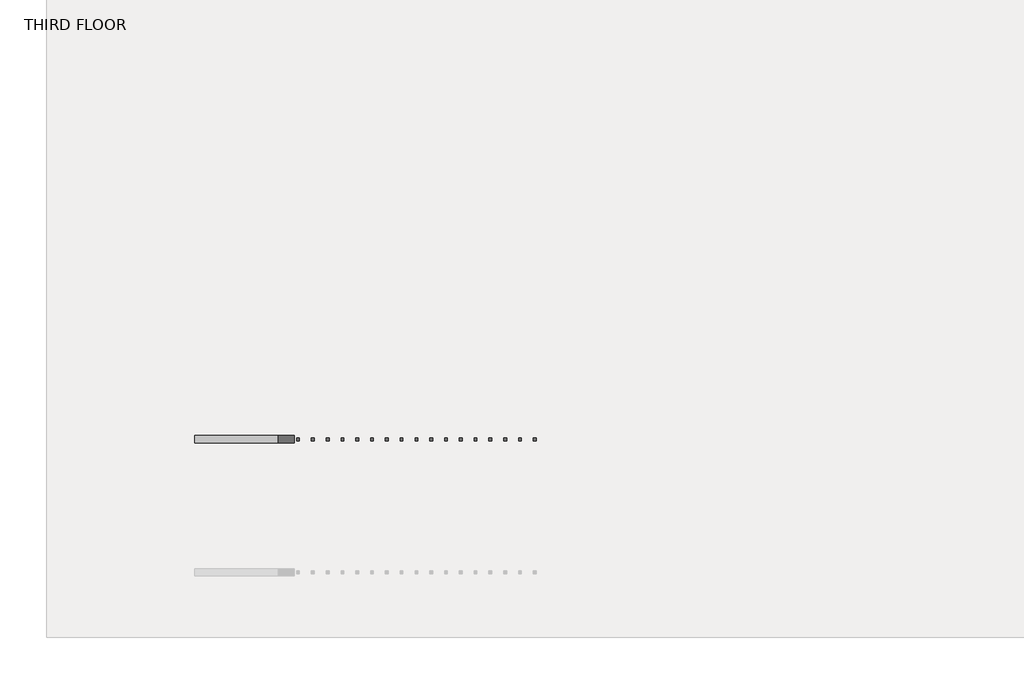
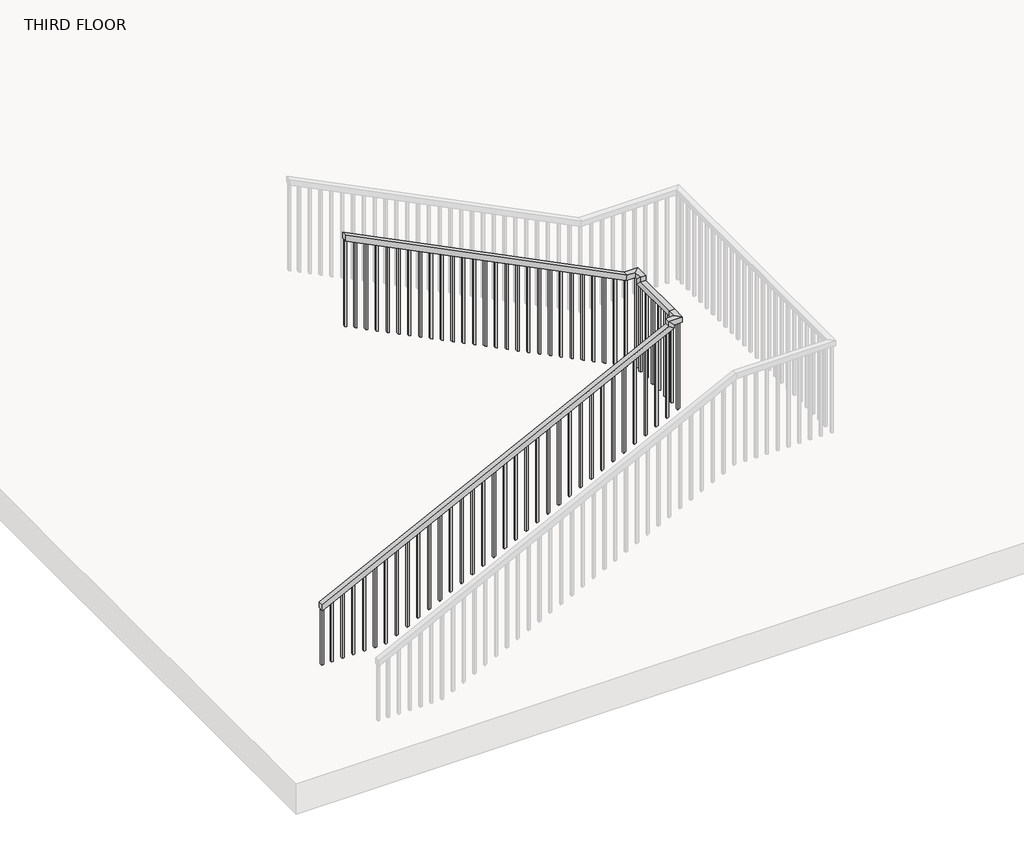
# One storey, part 2 of 2: 1 railing.
"""IFC4 building model written with IfcOpenShell, lengths in millimetres."""

from ifc_helpers import new_model, si_unit, frame, origin, place, context, project, spatial, polyline, outline, extrude, faceted_brep, element, save

model = new_model("IFC4")

# Units and contexts
model_context = context("Model", 3, world=origin())
ifc_project = project(units=[si_unit("LENGTHUNIT", "METRE", prefix="MILLI")], contexts=[model_context])

# Site, building, storey
site = spatial("IfcSite", under=ifc_project)
building = spatial("IfcBuilding", under=site)
storey = spatial("IfcBuildingStorey", under=building, Name="THIRD FLOOR", Elevation=9144.0)

# Railing
placement = place(None, origin())
element("IfcRailing", 1, ObjectType="Handrail - Rectangular", at=placement, inside=storey, context=model_context, shape_type="SolidModel", body=[
    faceted_brep([(-8362.2800418, -4455.7090076, 10058.4), (-8362.2800418, -4455.7090076, 10001.6038734), (-8362.2800418, -4506.5090076, 10001.6038734), (-8362.2800418, -4506.5090076, 10058.4), (-5111.0800418, -4455.7090076, 11684.0), (-5060.2800418, -4455.7090076, 11652.6038734), (-5060.2800418, -4506.5090076, 11652.6038734), (-5111.0800418, -4506.5090076, 11684.0), (-5111.0800418, -4455.7090076, 11734.8), (-5060.2800418, -4455.7090076, 11684.0), (-5060.2800418, -4506.5090076, 11684.0), (-5111.0800418, -4506.5090076, 11734.8), (-5034.8800418, -4455.7090076, 11734.8), (-5034.8800418, -4455.7090076, 11684.0), (-4984.0800418, -4506.5090076, 11684.0), (-4984.0800418, -4506.5090076, 11734.8), (-5034.8800418, -4379.5090076, 11734.8), (-5034.8800418, -4379.5090076, 11684.0), (-4984.0800418, -4379.5090076, 11684.0), (-4984.0800418, -4379.5090076, 11734.8), (-5034.8800418, -3907.7346494, 11734.8), (-5034.8800418, -3856.9346494, 11684.0), (-4984.0800418, -3856.9346494, 11684.0), (-4984.0800418, -3907.7346494, 11734.8), (-5034.8800418, -3907.7346494, 11785.6), (-5034.8800418, -3856.9346494, 11734.8), (-4984.0800418, -3856.9346494, 11734.8), (-4984.0800418, -3907.7346494, 11785.6), (-5034.8800418, -3831.5346494, 11785.6), (-5034.8800418, -3831.5346494, 11734.8), (-4984.0800418, -3780.7346494, 11734.8), (-4984.0800418, -3780.7346494, 11785.6), (-5111.0800418, -3831.5346494, 11785.6), (-5123.072295, -3831.5346494, 11734.8), (-5123.072295, -3780.7346494, 11734.8), (-5111.0800418, -3780.7346494, 11785.6), (-7752.6800418, -3831.5346494, 13106.4), (-7752.6800418, -3780.7346494, 13106.4), (-7752.6800418, -3780.7346494, 13049.6038734), (-7752.6800418, -3831.5346494, 13049.6038734)], [[[0, 1, 2, 3]], [[1, 0, 4, 5]], [[2, 1, 5, 6]], [[3, 2, 6, 7]], [[0, 3, 7, 4]], [[5, 4, 8, 9]], [[6, 5, 9, 10]], [[7, 6, 10, 11]], [[4, 7, 11, 8]], [[9, 8, 12, 13]], [[10, 9, 13, 14]], [[11, 10, 14, 15]], [[8, 11, 15, 12]], [[13, 12, 16, 17]], [[14, 13, 17, 18]], [[15, 14, 18, 19]], [[12, 15, 19, 16]], [[17, 16, 20, 21]], [[18, 17, 21, 22]], [[19, 18, 22, 23]], [[16, 19, 23, 20]], [[21, 20, 24, 25]], [[22, 21, 25, 26]], [[23, 22, 26, 27]], [[20, 23, 27, 24]], [[25, 24, 28, 29]], [[26, 25, 29, 30]], [[27, 26, 30, 31]], [[24, 27, 31, 28]], [[29, 28, 32, 33]], [[30, 29, 33, 34]], [[31, 30, 34, 35]], [[28, 31, 35, 32]], [[36, 37, 38, 39]], [[33, 32, 36, 39]], [[34, 33, 39, 38]], [[35, 34, 38, 37]], [[32, 35, 37, 36]]]),
    extrude(outline(polyline([(12994.0413734, -7641.5550418), (13003.5663734, -7660.6050418), (12145.9625, -7660.6050418), (12136.4375, -7641.5550418), (12994.0413734, -7641.5550418)])), frame((0.0, -3815.6596494, 0.0), z_axis=(0.0, 1.0, 0.0), x_axis=(0.0, 0.0, 1.0)), (0.0, 0.0, 1.0), 19.05),
    extrude(outline(polyline([(12943.2413734, -7539.9550418), (12952.7663734, -7559.0050418), (12095.1625, -7559.0050418), (12085.6375, -7539.9550418), (12943.2413734, -7539.9550418)])), frame((0.0, -3815.6596494, 0.0), z_axis=(0.0, 1.0, 0.0), x_axis=(0.0, 0.0, 1.0)), (0.0, 0.0, 1.0), 19.05),
    extrude(outline(polyline([(12892.4413734, -7438.3550418), (12901.9663734, -7457.4050418), (12044.3625, -7457.4050418), (12034.8375, -7438.3550418), (12892.4413734, -7438.3550418)])), frame((0.0, -3815.6596494, 0.0), z_axis=(0.0, 1.0, 0.0), x_axis=(0.0, 0.0, 1.0)), (0.0, 0.0, 1.0), 19.05),
    extrude(outline(polyline([(12841.6413734, -7336.7550418), (12851.1663734, -7355.8050418), (11993.5625, -7355.8050418), (11984.0375, -7336.7550418), (12841.6413734, -7336.7550418)])), frame((0.0, -3815.6596494, 0.0), z_axis=(0.0, 1.0, 0.0), x_axis=(0.0, 0.0, 1.0)), (0.0, 0.0, 1.0), 19.05),
    extrude(outline(polyline([(12790.8413734, -7235.1550418), (12800.3663734, -7254.2050418), (11942.7625, -7254.2050418), (11933.2375, -7235.1550418), (12790.8413734, -7235.1550418)])), frame((0.0, -3815.6596494, 0.0), z_axis=(0.0, 1.0, 0.0), x_axis=(0.0, 0.0, 1.0)), (0.0, 0.0, 1.0), 19.05),
    extrude(outline(polyline([(12740.0413734, -7133.5550418), (12749.5663734, -7152.6050418), (11891.9625, -7152.6050418), (11882.4375, -7133.5550418), (12740.0413734, -7133.5550418)])), frame((0.0, -3815.6596494, 0.0), z_axis=(0.0, 1.0, 0.0), x_axis=(0.0, 0.0, 1.0)), (0.0, 0.0, 1.0), 19.05),
    extrude(outline(polyline([(12689.2413734, -7031.9550418), (12698.7663734, -7051.0050418), (11841.1625, -7051.0050418), (11831.6375, -7031.9550418), (12689.2413734, -7031.9550418)])), frame((0.0, -3815.6596494, 0.0), z_axis=(0.0, 1.0, 0.0), x_axis=(0.0, 0.0, 1.0)), (0.0, 0.0, 1.0), 19.05),
    extrude(outline(polyline([(12638.4413734, -6930.3550418), (12647.9663734, -6949.4050418), (11790.3625, -6949.4050418), (11780.8375, -6930.3550418), (12638.4413734, -6930.3550418)])), frame((0.0, -3815.6596494, 0.0), z_axis=(0.0, 1.0, 0.0), x_axis=(0.0, 0.0, 1.0)), (0.0, 0.0, 1.0), 19.05),
    extrude(outline(polyline([(12587.6413734, -6828.7550418), (12597.1663734, -6847.8050418), (11739.5625, -6847.8050418), (11730.0375, -6828.7550418), (12587.6413734, -6828.7550418)])), frame((0.0, -3815.6596494, 0.0), z_axis=(0.0, 1.0, 0.0), x_axis=(0.0, 0.0, 1.0)), (0.0, 0.0, 1.0), 19.05),
    extrude(outline(polyline([(12536.8413734, -6727.1550418), (12546.3663734, -6746.2050418), (11688.7625, -6746.2050418), (11679.2375, -6727.1550418), (12536.8413734, -6727.1550418)])), frame((0.0, -3815.6596494, 0.0), z_axis=(0.0, 1.0, 0.0), x_axis=(0.0, 0.0, 1.0)), (0.0, 0.0, 1.0), 19.05),
    extrude(outline(polyline([(12486.0413734, -6625.5550418), (12495.5663734, -6644.6050418), (11637.9625, -6644.6050418), (11628.4375, -6625.5550418), (12486.0413734, -6625.5550418)])), frame((0.0, -3815.6596494, 0.0), z_axis=(0.0, 1.0, 0.0), x_axis=(0.0, 0.0, 1.0)), (0.0, 0.0, 1.0), 19.05),
    extrude(outline(polyline([(12435.2413734, -6523.9550418), (12444.7663734, -6543.0050418), (11587.1625, -6543.0050418), (11577.6375, -6523.9550418), (12435.2413734, -6523.9550418)])), frame((0.0, -3815.6596494, 0.0), z_axis=(0.0, 1.0, 0.0), x_axis=(0.0, 0.0, 1.0)), (0.0, 0.0, 1.0), 19.05),
    extrude(outline(polyline([(12384.4413734, -6422.3550418), (12393.9663734, -6441.4050418), (11536.3625, -6441.4050418), (11526.8375, -6422.3550418), (12384.4413734, -6422.3550418)])), frame((0.0, -3815.6596494, 0.0), z_axis=(0.0, 1.0, 0.0), x_axis=(0.0, 0.0, 1.0)), (0.0, 0.0, 1.0), 19.05),
    extrude(outline(polyline([(12333.6413734, -6320.7550418), (12343.1663734, -6339.8050418), (11485.5625, -6339.8050418), (11476.0375, -6320.7550418), (12333.6413734, -6320.7550418)])), frame((0.0, -3815.6596494, 0.0), z_axis=(0.0, 1.0, 0.0), x_axis=(0.0, 0.0, 1.0)), (0.0, 0.0, 1.0), 19.05),
    extrude(outline(polyline([(12282.8413734, -6219.1550418), (12292.3663734, -6238.2050418), (11434.7625, -6238.2050418), (11425.2375, -6219.1550418), (12282.8413734, -6219.1550418)])), frame((0.0, -3815.6596494, 0.0), z_axis=(0.0, 1.0, 0.0), x_axis=(0.0, 0.0, 1.0)), (0.0, 0.0, 1.0), 19.05),
    extrude(outline(polyline([(12232.0413734, -6117.5550418), (12241.5663734, -6136.6050418), (11383.9625, -6136.6050418), (11374.4375, -6117.5550418), (12232.0413734, -6117.5550418)])), frame((0.0, -3815.6596494, 0.0), z_axis=(0.0, 1.0, 0.0), x_axis=(0.0, 0.0, 1.0)), (0.0, 0.0, 1.0), 19.05),
    extrude(outline(polyline([(12181.2413734, -6015.9550418), (12190.7663734, -6035.0050418), (11333.1625, -6035.0050418), (11323.6375, -6015.9550418), (12181.2413734, -6015.9550418)])), frame((0.0, -3815.6596494, 0.0), z_axis=(0.0, 1.0, 0.0), x_axis=(0.0, 0.0, 1.0)), (0.0, 0.0, 1.0), 19.05),
    extrude(outline(polyline([(12130.4413734, -5914.3550418), (12139.9663734, -5933.4050418), (11282.3625, -5933.4050418), (11272.8375, -5914.3550418), (12130.4413734, -5914.3550418)])), frame((0.0, -3815.6596494, 0.0), z_axis=(0.0, 1.0, 0.0), x_axis=(0.0, 0.0, 1.0)), (0.0, 0.0, 1.0), 19.05),
    extrude(outline(polyline([(12079.6413734, -5812.7550418), (12089.1663734, -5831.8050418), (11231.5625, -5831.8050418), (11222.0375, -5812.7550418), (12079.6413734, -5812.7550418)])), frame((0.0, -3815.6596494, 0.0), z_axis=(0.0, 1.0, 0.0), x_axis=(0.0, 0.0, 1.0)), (0.0, 0.0, 1.0), 19.05),
    extrude(outline(polyline([(12028.8413734, -5711.1550418), (12038.3663734, -5730.2050418), (11180.7625, -5730.2050418), (11171.2375, -5711.1550418), (12028.8413734, -5711.1550418)])), frame((0.0, -3815.6596494, 0.0), z_axis=(0.0, 1.0, 0.0), x_axis=(0.0, 0.0, 1.0)), (0.0, 0.0, 1.0), 19.05),
    extrude(outline(polyline([(11978.0413734, -5609.5550418), (11987.5663734, -5628.6050418), (11129.9625, -5628.6050418), (11120.4375, -5609.5550418), (11978.0413734, -5609.5550418)])), frame((0.0, -3815.6596494, 0.0), z_axis=(0.0, 1.0, 0.0), x_axis=(0.0, 0.0, 1.0)), (0.0, 0.0, 1.0), 19.05),
    extrude(outline(polyline([(11927.2413734, -5507.9550418), (11936.7663734, -5527.0050418), (11079.1625, -5527.0050418), (11069.6375, -5507.9550418), (11927.2413734, -5507.9550418)])), frame((0.0, -3815.6596494, 0.0), z_axis=(0.0, 1.0, 0.0), x_axis=(0.0, 0.0, 1.0)), (0.0, 0.0, 1.0), 19.05),
    extrude(outline(polyline([(11876.4413734, -5406.3550418), (11885.9663734, -5425.4050418), (11028.3625, -5425.4050418), (11018.8375, -5406.3550418), (11876.4413734, -5406.3550418)])), frame((0.0, -3815.6596494, 0.0), z_axis=(0.0, 1.0, 0.0), x_axis=(0.0, 0.0, 1.0)), (0.0, 0.0, 1.0), 19.05),
    extrude(outline(polyline([(11825.6413734, -5304.7550418), (11835.1663734, -5323.8050418), (10977.5625, -5323.8050418), (10968.0375, -5304.7550418), (11825.6413734, -5304.7550418)])), frame((0.0, -3815.6596494, 0.0), z_axis=(0.0, 1.0, 0.0), x_axis=(0.0, 0.0, 1.0)), (0.0, 0.0, 1.0), 19.05),
    extrude(outline(polyline([(11774.8413734, -5203.1550418), (11784.3663734, -5222.2050418), (10926.7625, -5222.2050418), (10917.2375, -5203.1550418), (11774.8413734, -5203.1550418)])), frame((0.0, -3815.6596494, 0.0), z_axis=(0.0, 1.0, 0.0), x_axis=(0.0, 0.0, 1.0)), (0.0, 0.0, 1.0), 19.05),
    extrude(outline(polyline([(11734.8, -5101.5550418), (11734.8, -5120.6050418), (10875.9625, -5120.6050418), (10866.4375, -5101.5550418), (11734.8, -5101.5550418)])), frame((0.0, -3815.6596494, 0.0), z_axis=(0.0, 1.0, 0.0), x_axis=(0.0, 0.0, 1.0)), (0.0, 0.0, 1.0), 19.05),
    extrude(outline(polyline([(-4999.9550418, -3881.0340076), (-5019.0050418, -3881.0340076), (-5019.0050418, -3861.9840076), (-4999.9550418, -3861.9840076), (-4999.9550418, -3881.0340076)])), frame((0.0, 0.0, 10820.4), z_axis=(0.0, 0.0, 1.0), x_axis=(1.0, 0.0, 0.0)), (0.0, 0.0, 1.0), 863.6),
    extrude(outline(polyline([(-4999.9550418, -3982.6340076), (-5019.0050418, -3982.6340076), (-5019.0050418, -3963.5840076), (-4999.9550418, -3963.5840076), (-4999.9550418, -3982.6340076)])), frame((0.0, 0.0, 10820.4), z_axis=(0.0, 0.0, 1.0), x_axis=(1.0, 0.0, 0.0)), (0.0, 0.0, 1.0), 863.6),
    extrude(outline(polyline([(-4999.9550418, -4084.2340076), (-5019.0050418, -4084.2340076), (-5019.0050418, -4065.1840076), (-4999.9550418, -4065.1840076), (-4999.9550418, -4084.2340076)])), frame((0.0, 0.0, 10820.4), z_axis=(0.0, 0.0, 1.0), x_axis=(1.0, 0.0, 0.0)), (0.0, 0.0, 1.0), 863.6),
    extrude(outline(polyline([(-4999.9550418, -4185.8340076), (-5019.0050418, -4185.8340076), (-5019.0050418, -4166.7840076), (-4999.9550418, -4166.7840076), (-4999.9550418, -4185.8340076)])), frame((0.0, 0.0, 10820.4), z_axis=(0.0, 0.0, 1.0), x_axis=(1.0, 0.0, 0.0)), (0.0, 0.0, 1.0), 863.6),
    extrude(outline(polyline([(-4999.9550418, -4287.4340076), (-5019.0050418, -4287.4340076), (-5019.0050418, -4268.3840076), (-4999.9550418, -4268.3840076), (-4999.9550418, -4287.4340076)])), frame((0.0, 0.0, 10820.4), z_axis=(0.0, 0.0, 1.0), x_axis=(1.0, 0.0, 0.0)), (0.0, 0.0, 1.0), 863.6),
    extrude(outline(polyline([(-4999.9550418, -4389.0340076), (-5019.0050418, -4389.0340076), (-5019.0050418, -4369.9840076), (-4999.9550418, -4369.9840076), (-4999.9550418, -4389.0340076)])), frame((0.0, 0.0, 10820.4), z_axis=(0.0, 0.0, 1.0), x_axis=(1.0, 0.0, 0.0)), (0.0, 0.0, 1.0), 863.6),
    extrude(outline(polyline([(11631.9663734, -5101.5550418), (11622.4413734, -5120.6050418), (10764.8375, -5120.6050418), (10774.3625, -5101.5550418), (11631.9663734, -5101.5550418)])), frame((0.0, -4490.6340076, 0.0), z_axis=(0.0, 1.0, 0.0), x_axis=(0.0, 0.0, 1.0)), (0.0, 0.0, 1.0), 19.05),
    extrude(outline(polyline([(11581.1663734, -5203.1550418), (11571.6413734, -5222.2050418), (10714.0375, -5222.2050418), (10723.5625, -5203.1550418), (11581.1663734, -5203.1550418)])), frame((0.0, -4490.6340076, 0.0), z_axis=(0.0, 1.0, 0.0), x_axis=(0.0, 0.0, 1.0)), (0.0, 0.0, 1.0), 19.05),
    extrude(outline(polyline([(11530.3663734, -5304.7550418), (11520.8413734, -5323.8050418), (10663.2375, -5323.8050418), (10672.7625, -5304.7550418), (11530.3663734, -5304.7550418)])), frame((0.0, -4490.6340076, 0.0), z_axis=(0.0, 1.0, 0.0), x_axis=(0.0, 0.0, 1.0)), (0.0, 0.0, 1.0), 19.05),
    extrude(outline(polyline([(11479.5663734, -5406.3550418), (11470.0413734, -5425.4050418), (10612.4375, -5425.4050418), (10621.9625, -5406.3550418), (11479.5663734, -5406.3550418)])), frame((0.0, -4490.6340076, 0.0), z_axis=(0.0, 1.0, 0.0), x_axis=(0.0, 0.0, 1.0)), (0.0, 0.0, 1.0), 19.05),
    extrude(outline(polyline([(11428.7663734, -5507.9550418), (11419.2413734, -5527.0050418), (10561.6375, -5527.0050418), (10571.1625, -5507.9550418), (11428.7663734, -5507.9550418)])), frame((0.0, -4490.6340076, 0.0), z_axis=(0.0, 1.0, 0.0), x_axis=(0.0, 0.0, 1.0)), (0.0, 0.0, 1.0), 19.05),
    extrude(outline(polyline([(11377.9663734, -5609.5550418), (11368.4413734, -5628.6050418), (10510.8375, -5628.6050418), (10520.3625, -5609.5550418), (11377.9663734, -5609.5550418)])), frame((0.0, -4490.6340076, 0.0), z_axis=(0.0, 1.0, 0.0), x_axis=(0.0, 0.0, 1.0)), (0.0, 0.0, 1.0), 19.05),
    extrude(outline(polyline([(11327.1663734, -5711.1550418), (11317.6413734, -5730.2050418), (10460.0375, -5730.2050418), (10469.5625, -5711.1550418), (11327.1663734, -5711.1550418)])), frame((0.0, -4490.6340076, 0.0), z_axis=(0.0, 1.0, 0.0), x_axis=(0.0, 0.0, 1.0)), (0.0, 0.0, 1.0), 19.05),
    extrude(outline(polyline([(11276.3663734, -5812.7550418), (11266.8413734, -5831.8050418), (10409.2375, -5831.8050418), (10418.7625, -5812.7550418), (11276.3663734, -5812.7550418)])), frame((0.0, -4490.6340076, 0.0), z_axis=(0.0, 1.0, 0.0), x_axis=(0.0, 0.0, 1.0)), (0.0, 0.0, 1.0), 19.05),
    extrude(outline(polyline([(11225.5663734, -5914.3550418), (11216.0413734, -5933.4050418), (10358.4375, -5933.4050418), (10367.9625, -5914.3550418), (11225.5663734, -5914.3550418)])), frame((0.0, -4490.6340076, 0.0), z_axis=(0.0, 1.0, 0.0), x_axis=(0.0, 0.0, 1.0)), (0.0, 0.0, 1.0), 19.05),
    extrude(outline(polyline([(11174.7663734, -6015.9550418), (11165.2413734, -6035.0050418), (10307.6375, -6035.0050418), (10317.1625, -6015.9550418), (11174.7663734, -6015.9550418)])), frame((0.0, -4490.6340076, 0.0), z_axis=(0.0, 1.0, 0.0), x_axis=(0.0, 0.0, 1.0)), (0.0, 0.0, 1.0), 19.05),
    extrude(outline(polyline([(11123.9663734, -6117.5550418), (11114.4413734, -6136.6050418), (10256.8375, -6136.6050418), (10266.3625, -6117.5550418), (11123.9663734, -6117.5550418)])), frame((0.0, -4490.6340076, 0.0), z_axis=(0.0, 1.0, 0.0), x_axis=(0.0, 0.0, 1.0)), (0.0, 0.0, 1.0), 19.05),
    extrude(outline(polyline([(11073.1663734, -6219.1550418), (11063.6413734, -6238.2050418), (10206.0375, -6238.2050418), (10215.5625, -6219.1550418), (11073.1663734, -6219.1550418)])), frame((0.0, -4490.6340076, 0.0), z_axis=(0.0, 1.0, 0.0), x_axis=(0.0, 0.0, 1.0)), (0.0, 0.0, 1.0), 19.05),
    extrude(outline(polyline([(11022.3663734, -6320.7550418), (11012.8413734, -6339.8050418), (10155.2375, -6339.8050418), (10164.7625, -6320.7550418), (11022.3663734, -6320.7550418)])), frame((0.0, -4490.6340076, 0.0), z_axis=(0.0, 1.0, 0.0), x_axis=(0.0, 0.0, 1.0)), (0.0, 0.0, 1.0), 19.05),
    extrude(outline(polyline([(10971.5663734, -6422.3550418), (10962.0413734, -6441.4050418), (10104.4375, -6441.4050418), (10113.9625, -6422.3550418), (10971.5663734, -6422.3550418)])), frame((0.0, -4490.6340076, 0.0), z_axis=(0.0, 1.0, 0.0), x_axis=(0.0, 0.0, 1.0)), (0.0, 0.0, 1.0), 19.05),
    extrude(outline(polyline([(10920.7663734, -6523.9550418), (10911.2413734, -6543.0050418), (10053.6375, -6543.0050418), (10063.1625, -6523.9550418), (10920.7663734, -6523.9550418)])), frame((0.0, -4490.6340076, 0.0), z_axis=(0.0, 1.0, 0.0), x_axis=(0.0, 0.0, 1.0)), (0.0, 0.0, 1.0), 19.05),
    extrude(outline(polyline([(10869.9663734, -6625.5550418), (10860.4413734, -6644.6050418), (10002.8375, -6644.6050418), (10012.3625, -6625.5550418), (10869.9663734, -6625.5550418)])), frame((0.0, -4490.6340076, 0.0), z_axis=(0.0, 1.0, 0.0), x_axis=(0.0, 0.0, 1.0)), (0.0, 0.0, 1.0), 19.05),
    extrude(outline(polyline([(10819.1663734, -6727.1550418), (10809.6413734, -6746.2050418), (9952.0375, -6746.2050418), (9961.5625, -6727.1550418), (10819.1663734, -6727.1550418)])), frame((0.0, -4490.6340076, 0.0), z_axis=(0.0, 1.0, 0.0), x_axis=(0.0, 0.0, 1.0)), (0.0, 0.0, 1.0), 19.05),
    extrude(outline(polyline([(10768.3663734, -6828.7550418), (10758.8413734, -6847.8050418), (9901.2375, -6847.8050418), (9910.7625, -6828.7550418), (10768.3663734, -6828.7550418)])), frame((0.0, -4490.6340076, 0.0), z_axis=(0.0, 1.0, 0.0), x_axis=(0.0, 0.0, 1.0)), (0.0, 0.0, 1.0), 19.05),
    extrude(outline(polyline([(10717.5663734, -6930.3550418), (10708.0413734, -6949.4050418), (9850.4375, -6949.4050418), (9859.9625, -6930.3550418), (10717.5663734, -6930.3550418)])), frame((0.0, -4490.6340076, 0.0), z_axis=(0.0, 1.0, 0.0), x_axis=(0.0, 0.0, 1.0)), (0.0, 0.0, 1.0), 19.05),
    extrude(outline(polyline([(10666.7663734, -7031.9550418), (10657.2413734, -7051.0050418), (9799.6375, -7051.0050418), (9809.1625, -7031.9550418), (10666.7663734, -7031.9550418)])), frame((0.0, -4490.6340076, 0.0), z_axis=(0.0, 1.0, 0.0), x_axis=(0.0, 0.0, 1.0)), (0.0, 0.0, 1.0), 19.05),
    extrude(outline(polyline([(10615.9663734, -7133.5550418), (10606.4413734, -7152.6050418), (9748.8375, -7152.6050418), (9758.3625, -7133.5550418), (10615.9663734, -7133.5550418)])), frame((0.0, -4490.6340076, 0.0), z_axis=(0.0, 1.0, 0.0), x_axis=(0.0, 0.0, 1.0)), (0.0, 0.0, 1.0), 19.05),
    extrude(outline(polyline([(10565.1663734, -7235.1550418), (10555.6413734, -7254.2050418), (9698.0375, -7254.2050418), (9707.5625, -7235.1550418), (10565.1663734, -7235.1550418)])), frame((0.0, -4490.6340076, 0.0), z_axis=(0.0, 1.0, 0.0), x_axis=(0.0, 0.0, 1.0)), (0.0, 0.0, 1.0), 19.05),
    extrude(outline(polyline([(10514.3663734, -7336.7550418), (10504.8413734, -7355.8050418), (9647.2375, -7355.8050418), (9656.7625, -7336.7550418), (10514.3663734, -7336.7550418)])), frame((0.0, -4490.6340076, 0.0), z_axis=(0.0, 1.0, 0.0), x_axis=(0.0, 0.0, 1.0)), (0.0, 0.0, 1.0), 19.05),
    extrude(outline(polyline([(10463.5663734, -7438.3550418), (10454.0413734, -7457.4050418), (9596.4375, -7457.4050418), (9605.9625, -7438.3550418), (10463.5663734, -7438.3550418)])), frame((0.0, -4490.6340076, 0.0), z_axis=(0.0, 1.0, 0.0), x_axis=(0.0, 0.0, 1.0)), (0.0, 0.0, 1.0), 19.05),
    extrude(outline(polyline([(10412.7663734, -7539.9550418), (10403.2413734, -7559.0050418), (9545.6375, -7559.0050418), (9555.1625, -7539.9550418), (10412.7663734, -7539.9550418)])), frame((0.0, -4490.6340076, 0.0), z_axis=(0.0, 1.0, 0.0), x_axis=(0.0, 0.0, 1.0)), (0.0, 0.0, 1.0), 19.05),
    extrude(outline(polyline([(10361.9663734, -7641.5550418), (10352.4413734, -7660.6050418), (9494.8375, -7660.6050418), (9504.3625, -7641.5550418), (10361.9663734, -7641.5550418)])), frame((0.0, -4490.6340076, 0.0), z_axis=(0.0, 1.0, 0.0), x_axis=(0.0, 0.0, 1.0)), (0.0, 0.0, 1.0), 19.05),
    extrude(outline(polyline([(10311.1663734, -7743.1550418), (10301.6413734, -7762.2050418), (9444.0375, -7762.2050418), (9453.5625, -7743.1550418), (10311.1663734, -7743.1550418)])), frame((0.0, -4490.6340076, 0.0), z_axis=(0.0, 1.0, 0.0), x_axis=(0.0, 0.0, 1.0)), (0.0, 0.0, 1.0), 19.05),
    extrude(outline(polyline([(10260.3663734, -7844.7550418), (10250.8413734, -7863.8050418), (9393.2375, -7863.8050418), (9402.7625, -7844.7550418), (10260.3663734, -7844.7550418)])), frame((0.0, -4490.6340076, 0.0), z_axis=(0.0, 1.0, 0.0), x_axis=(0.0, 0.0, 1.0)), (0.0, 0.0, 1.0), 19.05),
    extrude(outline(polyline([(10209.5663734, -7946.3550418), (10200.0413734, -7965.4050418), (9342.4375, -7965.4050418), (9351.9625, -7946.3550418), (10209.5663734, -7946.3550418)])), frame((0.0, -4490.6340076, 0.0), z_axis=(0.0, 1.0, 0.0), x_axis=(0.0, 0.0, 1.0)), (0.0, 0.0, 1.0), 19.05),
    extrude(outline(polyline([(10158.7663734, -8047.9550418), (10149.2413734, -8067.0050418), (9291.6375, -8067.0050418), (9301.1625, -8047.9550418), (10158.7663734, -8047.9550418)])), frame((0.0, -4490.6340076, 0.0), z_axis=(0.0, 1.0, 0.0), x_axis=(0.0, 0.0, 1.0)), (0.0, 0.0, 1.0), 19.05),
    extrude(outline(polyline([(10107.9663734, -8149.5550418), (10098.4413734, -8168.6050418), (9240.8375, -8168.6050418), (9250.3625, -8149.5550418), (10107.9663734, -8149.5550418)])), frame((0.0, -4490.6340076, 0.0), z_axis=(0.0, 1.0, 0.0), x_axis=(0.0, 0.0, 1.0)), (0.0, 0.0, 1.0), 19.05),
    extrude(outline(polyline([(10057.1663734, -8251.1550418), (10047.6413734, -8270.2050418), (9190.0375, -8270.2050418), (9199.5625, -8251.1550418), (10057.1663734, -8251.1550418)])), frame((0.0, -4490.6340076, 0.0), z_axis=(0.0, 1.0, 0.0), x_axis=(0.0, 0.0, 1.0)), (0.0, 0.0, 1.0), 19.05),
    extrude(outline(polyline([(-4999.9550418, -3815.6596494), (-5019.0050418, -3815.6596494), (-5019.0050418, -3796.6096494), (-4999.9550418, -3796.6096494), (-4999.9550418, -3815.6596494)])), frame((0.0, 0.0, 10820.4), z_axis=(0.0, 0.0, 1.0), x_axis=(1.0, 0.0, 0.0)), (0.0, 0.0, 1.0), 914.4),
    extrude(outline(polyline([(11684.0, -4999.9550418), (11684.0, -5019.0050418), (10815.6375, -5019.0050418), (10825.1625, -4999.9550418), (11684.0, -4999.9550418)])), frame((0.0, -4490.6340076, 0.0), z_axis=(0.0, 1.0, 0.0), x_axis=(0.0, 0.0, 1.0)), (0.0, 0.0, 1.0), 19.05),
    extrude(outline(polyline([(13040.0788734, -7733.6300418), (13049.6038734, -7752.6800418), (12192.0, -7752.6800418), (12182.475, -7733.6300418), (13040.0788734, -7733.6300418)])), frame((0.0, -3815.6596494, 0.0), z_axis=(0.0, 1.0, 0.0), x_axis=(0.0, 0.0, 1.0)), (0.0, 0.0, 1.0), 19.05),
    extrude(outline(polyline([(10011.1288734, -8343.2300418), (10001.6038734, -8362.2800418), (9144.0, -8362.2800418), (9153.525, -8343.2300418), (10011.1288734, -8343.2300418)])), frame((0.0, -4490.6340076, 0.0), z_axis=(0.0, 1.0, 0.0), x_axis=(0.0, 0.0, 1.0)), (0.0, 0.0, 1.0), 19.05),
])

save(model, "model.ifc")

# Revit data of these elements
# Type "Handrail - Rectangular"
#   Assembly Code = "C2010400"
#   built-in parameter 1008612 = 0.0416667 (stored number, unit not read)
#   built-in parameter 1008611 = 0.0416667 (stored number, unit not read)
#   built-in parameter 1008609 = 0.333333 (stored number, unit not read)
#   built-in parameter 1008604 = 0.166667 (stored number, unit not read)
#   built-in parameter 1008603 = 0.166667 (stored number, unit not read)
#   Railing Height = 3' - 0"
#   built-in parameter 1008630 = 2
#   built-in parameter 1008610 = 2
#   built-in parameter 1008618 = Baluster - Square : 3/4"
# Element 1 (IfcRailing, "Handrail - Rectangular")
#   Phase Created = New Construction
